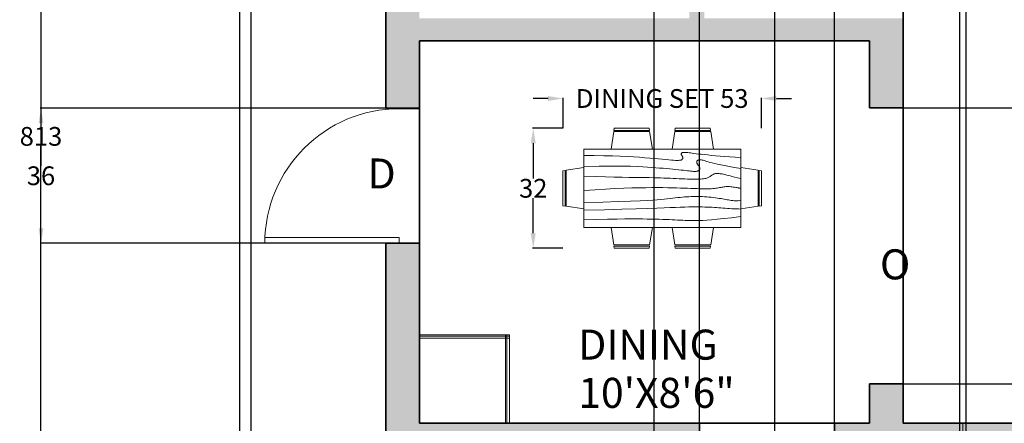
# Model space of a CAD drawing. Units: inches. Extents: x 460 to 1030, y -658 to 271.
# Tile 3 of 10: x 465 to 728, y -282 to -174. Entities that reach past the tile are written whole.
import ezdxf

# ---------------------------------------------------------------- set-up
doc = ezdxf.new("R2010")
doc.units = ezdxf.units.IN
doc.header["$MEASUREMENT"] = 0
for name, color, linetype, lineweight in [('A-ANNO-DIMS', 2, 'Continuous', 18), ('A-ANNO-TEXT', 7, 'Continuous', 18), ('A-AREA-IDEN', 7, 'Continuous', 25), ('A-DOOR', 3, 'Continuous', 20), ('A-FLOR-CASE', 9, 'Continuous', 18), ('A-FURN', 8, 'Continuous', 18), ('A-GLAZ', 4, 'Continuous', 20), ('A-GLAZ-PATT', 4, 'Continuous', 13), ('A-WALL', 7, 'Continuous', 35), ('A-WALL-PATT', 5, 'Continuous', 13), ('C-PROP', 7, 'Continuous', 25)]:
    doc.layers.add(name, color=color, linetype=linetype, lineweight=lineweight)
doc.styles.get("Standard").update_dxf_attribs({"font": 'arial.ttf'})
doc.dimstyles.get("Standard").update_dxf_attribs({"dimtxt": 5, "dimasz": 4, "dimexe": 0.18, "dimexo": 0.0625, "dimgap": 0.09, "dimtad": 0, "dimtih": 1, "dimtoh": 1, "dimdec": 1, "dimzin": 0, "dimdsep": 46, "dimlunit": 4, "dimtxsty": 'Standard', "dimcen": 0.09, "dimadec": 0, "dimazin": 0, "dimtfac": 1, "dimtdec": 1, "dimtofl": 0, "dimtmove": 0, "dimatfit": 3, "dimfxl": 1, "dimtolj": 1, "dimtzin": 0, "dimarcsym": 0})

# ---------------------------------------------------------------- blocks, each defined once
blk = doc.blocks.new('*U2')
for p, q in [((0, 0), (0, -6)), ((40, 0), (40, -6))]:
    blk.add_line(p, q)
blk.add_lwpolyline([(0, 0), (0, 40), (1.75, 40), (1.75, 0)], close=True)
blk.add_arc((0, 0), 40, 0, 90)
blk = doc.blocks.new('Dining Set - 36 x 72 in.')
for p, q in [((-22, 27.5), (-22.1562, 26.50042)), ((-22, 27.5), (-6, 27.5)), ((-5.8437, 26.49966), (-6, 27.5)), ((6, 27.5), (5.8438, 26.50042)), ((6, 27.5), (22, 27.5)), ((22.1563, 26.49966), (22, 27.5)), ((-22.2343, 26.00059), (-23.4847, 17.99762)), ((-22.2304, 26), (-5.7608, 26)), ((-5.8416, 26.5), (-22.1534, 26.5)), ((-4.5152, 17.99762), (-5.7655, 25.99926)), ((5.7657, 26.00059), (4.5153, 17.99762)), ((5.7696, 26), (22.2392, 26)), ((22.1584, 26.5), (5.8466, 26.5)), ((23.4848, 17.99762), (22.2345, 25.99926)), ((36, 18), (-36, 18)), ((-36, 18), (-36, -18)), ((36, -18), (36, 18)), ((-44.0006, 8.23428), (-35.9976, 9.48474)), ((44.0006, 8.23428), (35.9976, 9.48474)), ((-45.5, 8), (-44.5004, 8.15617)), ((-45.5, 8), (-45.5, -8)), ((-44.5, -8.15843), (-44.5, 8.15338)), ((-44, 8.23041), (-44, -8.23915)), ((44, 8.23041), (44, -8.23915)), ((44.5, -8.15843), (44.5, 8.15338)), ((45.5, 8), (44.5005, 8.15617)), ((45.5, 8), (45.5, -8)), ((-44.4997, -8.15631), (-45.5, -8)), ((-35.9976, -9.48476), (-43.9993, -8.2345)), ((35.9976, -9.48476), (43.9993, -8.2345)), ((44.4997, -8.15631), (45.5, -8)), ((-36, -18), (36, -18)), ((-22.2343, -26.0006), (-23.4847, -17.99762)), ((-4.5152, -17.99762), (-5.7655, -25.99928)), ((5.7657, -26.0006), (4.5153, -17.99762)), ((23.4848, -17.99762), (22.2345, -25.99928)), ((-22.2304, -26), (-5.7608, -26)), ((-22, -27.5), (-22.1562, -26.50044)), ((-5.8416, -26.5), (-22.1534, -26.5)), ((-5.8437, -26.49967), (-6, -27.5)), ((5.7696, -26), (22.2392, -26)), ((6, -27.5), (5.8438, -26.50044)), ((22.1584, -26.5), (5.8466, -26.5)), ((22.1563, -26.49967), (22, -27.5)), ((-22, -27.5), (-6, -27.5)), ((6, -27.5), (22, -27.5))]:
    blk.add_line(p, q)
for points in [[(-36, 15), (-31.1772, 14.97754), (-26.8079, 14.91406), (-22.8538, 14.81543), (-19.276, 14.6875), (-16.0362, 14.53613), (-13.0957, 14.36718), (-10.4159, 14.18652), (-7.9583, 14), (-5.6904, 13.81315), (-3.6035, 13.63021), (-1.6954, 13.45508), (0.0365, 13.29166), (1.5945, 13.14388), (2.9811, 13.01562), (4.1988, 12.9108), (5.25, 12.83333), (6.1393, 12.78613), (6.8802, 12.76823), (7.4883, 12.77767), (7.9792, 12.8125), (8.3685, 12.87077), (8.6719, 12.95052), (8.9049, 13.0498), (9.0833, 13.16666), (9.2205, 13.29899), (9.3216, 13.44401), (9.3895, 13.59879), (9.4271, 13.76041), (9.4373, 13.92594), (9.4232, 14.09245), (9.3875, 14.257), (9.3333, 14.41666), (9.2638, 14.56917), (9.1836, 14.71484), (9.0975, 14.85465), (9.0104, 14.98958), (8.9272, 15.1206), (8.8529, 15.2487), (8.7922, 15.37483), (8.75, 15.5), (8.7305, 15.62467), (8.7344, 15.74739), (8.7617, 15.86621), (8.8125, 15.97916), (8.8867, 16.08431), (8.9844, 16.17968), (9.1055, 16.26334), (9.25, 16.33333), (9.4189, 16.38802), (9.6172, 16.42708), (9.8506, 16.45052), (10.125, 16.45833), (10.4463, 16.45052), (10.8203, 16.42708), (11.2529, 16.38802), (11.75, 16.33333), (12.3184, 16.26318), (12.9694, 16.17838), (13.7151, 16.07991), (14.5677, 15.96875), (15.5395, 15.84586), (16.6426, 15.71224), (17.8893, 15.56884), (19.2917, 15.41666), (20.859, 15.25667), (22.5879, 15.08984), (24.4721, 14.91715), (26.5052, 14.73958), (28.6809, 14.5581), (30.9929, 14.3737), (33.4347, 14.18733), (36, 14)], [(-36, 10), (-28.9766, 10.14274), (-23.1725, 10.20442), (-18.4241, 10.19775), (-14.5677, 10.13541), (-11.4399, 10.03011), (-8.877, 9.89453), (-6.7154, 9.74137), (-4.7917, 9.58333), (-2.9698, 9.43082), (-1.2246, 9.28515), (0.4415, 9.14534), (2.026, 9.01041), (3.5266, 8.87939), (4.9408, 8.7513), (6.266, 8.62516), (7.5, 8.5), (8.6411, 8.37549), (9.6914, 8.2539), (10.6538, 8.13818), (11.5312, 8.03125), (12.3267, 7.93603), (13.043, 7.85547), (13.6831, 7.79248), (14.25, 7.75), (14.7471, 7.7303), (15.1797, 7.73307), (15.5537, 7.75732), (15.875, 7.80208), (16.1494, 7.86637), (16.3828, 7.94922), (16.5811, 8.04964), (16.75, 8.16666), (16.8944, 8.29915), (17.0143, 8.44531), (17.1089, 8.60319), (17.1771, 8.77083), (17.218, 8.94629), (17.2305, 9.1276), (17.2137, 9.31282), (17.1667, 9.5), (17.0895, 9.6875), (16.987, 9.875), (16.8649, 10.0625), (16.7292, 10.25), (16.5856, 10.4375), (16.4401, 10.625), (16.2985, 10.8125), (16.1667, 11), (16.05, 11.18733), (15.9518, 11.3737), (15.8752, 11.5581), (15.8229, 11.73958), (15.798, 11.91715), (15.8034, 12.08984), (15.842, 12.25667), (15.9167, 12.41666), (16.0295, 12.56836), (16.1784, 12.70833), (16.3605, 12.83268), (16.5729, 12.9375), (16.8127, 13.01888), (17.0768, 13.07291), (17.3625, 13.0957), (17.6667, 13.08333), (17.9894, 13.03312), (18.3418, 12.94726), (18.7382, 12.82918), (19.1927, 12.68229), (19.7195, 12.51001), (20.3327, 12.31575), (21.0465, 12.10294), (21.875, 11.875), (22.8357, 11.63354), (23.959, 11.37304), (25.2786, 11.08618), (26.8282, 10.76562), (28.6414, 10.40405), (30.752, 9.99414), (33.1936, 9.52856), (36, 9)], [(-36, 5.5), (-30.7157, 5.3348), (-26.069, 5.20963), (-21.9946, 5.11767), (-18.4271, 5.05208), (-15.3009, 5.00602), (-12.5508, 4.97265), (-10.1112, 4.94515), (-7.9167, 4.91666), (-5.909, 4.88167), (-4.0586, 4.83984), (-2.3429, 4.79215), (-0.7396, 4.73958), (0.7739, 4.6831), (2.22, 4.6237), (3.6213, 4.56233), (5, 4.5), (6.373, 4.43782), (7.7344, 4.3776), (9.0723, 4.32129), (10.375, 4.27083), (11.6309, 4.22819), (12.8281, 4.19531), (13.9551, 4.17415), (15, 4.16666), (15.954, 4.17448), (16.819, 4.19791), (17.6001, 4.23698), (18.3021, 4.29166), (18.9299, 4.36198), (19.4883, 4.44791), (19.9823, 4.54948), (20.4167, 4.66666), (20.7969, 4.79899), (21.1302, 4.94401), (21.4245, 5.09879), (21.6875, 5.26041), (21.9271, 5.42594), (22.1511, 5.59245), (22.3672, 5.757), (22.5834, 5.91666), (22.8065, 6.06868), (23.0404, 6.21093), (23.2879, 6.34147), (23.5521, 6.45833), (23.8358, 6.55957), (24.142, 6.64323), (24.4735, 6.70735), (24.8334, 6.75), (25.2235, 6.76969), (25.642, 6.76692), (26.0858, 6.74267), (26.5521, 6.69791), (27.0379, 6.63362), (27.5404, 6.55078), (28.0565, 6.45036), (28.5834, 6.33333), (29.1242, 6.19987), (29.7071, 6.04687), (30.3661, 5.87044), (31.1354, 5.66666), (32.0493, 5.43164), (33.142, 5.16146), (34.4475, 4.85221), (36, 4.5)], [(-36, -1), (-30.7915, -0.6591), (-26.0195, -0.38216), (-21.6519, -0.16284), (-17.6563, 0.00521), (-14.0005, 0.12833), (-10.6523, 0.21289), (-7.5796, 0.26522), (-4.75, 0.29166), (-2.134, 0.29793), (0.2878, 0.28711), (2.5317, 0.26163), (4.6146, 0.22396), (6.5529, 0.17651), (8.3633, 0.12174), (10.0623, 0.06209), (11.6667, 0), (13.1899, -0.06201), (14.6341, -0.1211), (15.9982, -0.17432), (17.2813, -0.21875), (18.4823, -0.25147), (19.6003, -0.26953), (20.6343, -0.27002), (21.5834, -0.25), (22.4481, -0.20768), (23.2357, -0.14584), (23.9549, -0.06836), (24.6146, 0.02083), (25.2235, 0.11784), (25.7904, 0.21875), (26.3241, 0.31966), (26.8334, 0.41666), (27.3265, 0.50618), (27.8099, 0.58593), (28.2894, 0.65397), (28.7709, 0.70833), (29.2601, 0.74707), (29.763, 0.76823), (30.2855, 0.76985), (30.8334, 0.75), (31.4088, 0.70784), (31.9994, 0.64713), (32.589, 0.57275), (33.1615, 0.48958), (33.7008, 0.4025), (34.1908, 0.3164), (34.6153, 0.23616), (34.9584, 0.16666), (35.2099, 0.11165), (35.3848, 0.07031), (35.504, 0.04069), (35.5886, 0.02083), (35.6594, 0.00879), (35.7377, 0.0026), (35.8442, 0.00032), (36, 0)], [(-36, -6.5), (-27.1843, -6.31267), (-20.084, -6.1263), (-14.469, -5.9419), (-10.1094, -5.76042), (-6.7752, -5.58285), (-4.2363, -5.41016), (-2.2629, -5.24333), (-0.625, -5.08334), (0.8708, -4.93099), (2.2715, -4.78646), (3.5872, -4.64974), (4.8281, -4.52084), (6.0046, -4.39974), (7.127, -4.28646), (8.2053, -4.18099), (9.25, -4.08334), (10.2705, -3.99382), (11.2734, -3.91407), (12.2647, -3.84603), (13.25, -3.79167), (14.2354, -3.75293), (15.2266, -3.73177), (16.2295, -3.73015), (17.25, -3.75), (18.2912, -3.79248), (19.3451, -3.85547), (20.4009, -3.93604), (21.4479, -4.03125), (22.4754, -4.13819), (23.4727, -4.25391), (24.4289, -4.37549), (25.3334, -4.5), (26.1785, -4.62492), (26.9694, -4.74935), (27.7145, -4.87281), (28.4219, -4.99479), (29.1, -5.11483), (29.7572, -5.23242), (30.4016, -5.34709), (31.0417, -5.45834), (31.6837, -5.56437), (32.3262, -5.65821), (32.9658, -5.73153), (33.599, -5.77604), (34.2224, -5.78345), (34.8327, -5.74545), (35.4264, -5.65373), (36, -5.5)], [(-36, -10), (-26.4022, -9.81299), (-18.4675, -9.62891), (-11.9839, -9.45069), (-6.7396, -9.28125), (-2.5226, -9.12354), (0.8789, -8.98047), (3.6769, -8.85498), (6.0833, -8.75), (8.2767, -8.66765), (10.3021, -8.60677), (12.1712, -8.56543), (13.8958, -8.54167), (15.4876, -8.53353), (16.9583, -8.53907), (18.3197, -8.55632), (19.5834, -8.58334), (20.7616, -8.61841), (21.8685, -8.66081), (22.9188, -8.71004), (23.9271, -8.76563), (24.9081, -8.82707), (25.8763, -8.89388), (26.8465, -8.96558), (27.8334, -9.04167), (28.8474, -9.12118), (29.8828, -9.20117), (30.93, -9.27824), (31.9792, -9.34896), (33.0205, -9.40991), (34.0443, -9.45768), (35.0407, -9.48885), (36, -9.5)], [(-36, -14.5), (-30.0881, -14.33513), (-25.0332, -14.21224), (-20.7312, -14.12647), (-17.0781, -14.07292), (-13.97, -14.04671), (-11.3027, -14.04297), (-8.9724, -14.05681), (-6.875, -14.08334), (-4.9224, -14.11833), (-3.0905, -14.16016), (-1.3709, -14.20785), (0.2448, -14.26042), (1.7647, -14.3169), (3.1973, -14.3763), (4.5507, -14.43767), (5.8333, -14.5), (7.0554, -14.5621), (8.235, -14.62175), (9.3922, -14.67652), (10.5469, -14.72396), (11.7192, -14.76164), (12.929, -14.78711), (14.1965, -14.79794), (15.5417, -14.79167), (16.9933, -14.76424), (18.6152, -14.70508), (20.4804, -14.60197), (22.6615, -14.44271), (25.2312, -14.21509), (28.2624, -13.9069), (31.8277, -13.50594), (36, -13)]]:
    blk.add_lwpolyline(points)
blk = doc.blocks.new('*D35')
at = {"layer": 'A-ANNO-DIMS', "color": 0, "lineweight": -2, "transparency": 16777216}
for p, q in [((606.08, -195.13), (602.08, -195.13)), ((610.08, -203.01), (610.08, -194.95)), ((663, -203.01), (663, -194.95)), ((667, -195.13), (671, -195.13))]:
    blk.add_line(p, q, dxfattribs=at)
at = {"layer": 'A-ANNO-DIMS', "color": 0, "transparency": 16777216}
for points in [[(606.08, -194.47), (606.08, -195.8), (610.08, -195.13)], [(667, -194.47), (667, -195.8), (663, -195.13)]]:
    blk.add_solid(points, dxfattribs=at)
at = {"layer": 'Defpoints', "color": 0, "transparency": 16777216}
for p in [(663, -195.13), (610.08, -203.07), (663, -203.07)]:
    blk.add_point(p, dxfattribs=at)
at = {"layer": 'A-ANNO-DIMS', "color": 0, "transparency": 16777216, "insert": (636.54, -195.13), "char_height": 5, "attachment_point": 5}
blk.add_mtext('\\A1;DINING SET 53', dxfattribs=at)
blk = doc.blocks.new('*D36')
at = {"layer": 'A-ANNO-DIMS', "color": 0, "lineweight": -2, "transparency": 16777216}
for p, q in [((610.02, -203.07), (601.96, -203.07)), ((602.14, -207.07), (602.14, -216.42)), ((602.14, -231.06), (602.14, -221.71)), ((610.02, -235.06), (601.96, -235.06))]:
    blk.add_line(p, q, dxfattribs=at)
at = {"layer": 'A-ANNO-DIMS', "color": 0, "transparency": 16777216}
for points in [[(601.47, -207.07), (602.81, -207.07), (602.14, -203.07)], [(601.47, -231.06), (602.81, -231.06), (602.14, -235.06)]]:
    blk.add_solid(points, dxfattribs=at)
at = {"layer": 'Defpoints', "color": 0, "transparency": 16777216}
for p in [(602.14, -203.07), (610.08, -203.07), (610.08, -235.06)]:
    blk.add_point(p, dxfattribs=at)
at = {"layer": 'A-ANNO-DIMS', "color": 0, "transparency": 16777216, "insert": (602.14, -219.07), "char_height": 5, "attachment_point": 5}
blk.add_mtext('\\A1;32', dxfattribs=at)
blk = doc.blocks.new('*D40')
at = {"layer": 'A-ANNO-DIMS', "color": 0, "lineweight": -2, "transparency": 16777216}
for p, q in [((523.73, 201.27), (470.68, 201.27)), ((470.86, 197.27), (470.86, -202.58)), ((470.86, -607.73), (470.86, -207.87)), ((523.73, -611.73), (470.68, -611.73))]:
    blk.add_line(p, q, dxfattribs=at)
at = {"layer": 'A-ANNO-DIMS', "color": 0, "transparency": 16777216}
for points in [[(470.19, 197.27), (471.52, 197.27), (470.86, 201.27)], [(470.19, -607.73), (471.52, -607.73), (470.86, -611.73)]]:
    blk.add_solid(points, dxfattribs=at)
at = {"layer": 'Defpoints', "color": 0, "transparency": 16777216}
for p in [(470.86, 201.27), (523.8, 201.27), (523.8, -611.73)]:
    blk.add_point(p, dxfattribs=at)
at = {"layer": 'A-ANNO-DIMS', "color": 0, "transparency": 16777216, "insert": (470.86, -205.23), "char_height": 5, "attachment_point": 5}
blk.add_mtext('\\A1;813', dxfattribs=at)
blk = doc.blocks.new('*D57')
at = {"layer": 'A-ANNO-DIMS', "color": 0, "lineweight": -2, "transparency": 16777216}
for p, q in [((717.53, -38.79), (717.53, -654.61)), ((741.59, -38.79), (741.59, -654.61)), ((713.53, -654.43), (709.53, -654.43)), ((745.59, -654.43), (749.59, -654.43))]:
    blk.add_line(p, q, dxfattribs=at)
at = {"layer": 'A-ANNO-DIMS', "color": 0, "transparency": 16777216}
for points in [[(713.53, -653.77), (713.53, -655.1), (717.53, -654.43)], [(745.59, -653.77), (745.59, -655.1), (741.59, -654.43)]]:
    blk.add_solid(points, dxfattribs=at)
at = {"layer": 'Defpoints', "color": 0, "transparency": 16777216}
for p in [(717.53, -38.73), (741.59, -38.73), (741.59, -654.43)]:
    blk.add_point(p, dxfattribs=at)
at = {"layer": 'A-ANNO-DIMS', "color": 0, "transparency": 16777216, "insert": (729.56, -654.43), "char_height": 5, "attachment_point": 5}
blk.add_mtext('\\A1;24.065', dxfattribs=at)
blk = doc.blocks.new('*D61')
at = {"layer": 'A-ANNO-DIMS', "color": 0, "lineweight": -2, "transparency": 16777216}
for p, q in [((646.47, -287.66), (646.47, 267.89)), ((682.47, -287.66), (682.47, 267.89)), ((650.47, 267.71), (660.81, 267.71)), ((678.47, 267.71), (668.14, 267.71))]:
    blk.add_line(p, q, dxfattribs=at)
at = {"layer": 'A-ANNO-DIMS', "color": 0, "transparency": 16777216}
for points in [[(650.47, 268.38), (650.47, 267.04), (646.47, 267.71)], [(678.47, 268.38), (678.47, 267.04), (682.47, 267.71)]]:
    blk.add_solid(points, dxfattribs=at)
at = {"layer": 'Defpoints', "color": 0, "transparency": 16777216}
for p in [(682.47, 267.71), (646.47, -287.73), (682.47, -287.73)]:
    blk.add_point(p, dxfattribs=at)
at = {"layer": 'A-ANNO-DIMS', "color": 0, "transparency": 16777216, "insert": (664.47, 267.71), "char_height": 5, "attachment_point": 5}
blk.add_mtext('\\A1;36', dxfattribs=at)
blk = doc.blocks.new('*D62')
at = {"layer": 'A-ANNO-DIMS', "color": 0, "lineweight": -2, "transparency": 16777216}
for p, q in [((700.86, -197.58), (1022.03, -197.58)), ((1021.85, -201.58), (1021.85, -231.74)), ((1021.85, -267.2), (1021.85, -237.03)), ((700.86, -271.2), (1022.03, -271.2))]:
    blk.add_line(p, q, dxfattribs=at)
at = {"layer": 'A-ANNO-DIMS', "color": 0, "transparency": 16777216}
for points in [[(1021.18, -201.58), (1022.51, -201.58), (1021.85, -197.58)], [(1021.18, -267.2), (1022.51, -267.2), (1021.85, -271.2)]]:
    blk.add_solid(points, dxfattribs=at)
at = {"layer": 'Defpoints', "color": 0, "transparency": 16777216}
for p in [(700.8, -197.58), (700.8, -271.2), (1021.85, -271.2)]:
    blk.add_point(p, dxfattribs=at)
at = {"layer": 'A-ANNO-DIMS', "color": 0, "transparency": 16777216, "insert": (1021.85, -234.39), "char_height": 5, "attachment_point": 5}
blk.add_mtext('\\A1;73.62', dxfattribs=at)
blk = doc.blocks.new('*D64')
at = {"layer": 'A-ANNO-DIMS', "color": 0, "lineweight": -2, "transparency": 16777216}
for p, q in [((562.73, -197.73), (470.68, -197.73)), ((470.86, -201.73), (470.86, -213.08)), ((470.86, -229.73), (470.86, -218.37)), ((562.73, -233.73), (470.68, -233.73))]:
    blk.add_line(p, q, dxfattribs=at)
at = {"layer": 'A-ANNO-DIMS', "color": 0, "transparency": 16777216}
for points in [[(470.19, -201.73), (471.52, -201.73), (470.86, -197.73)], [(470.19, -229.73), (471.52, -229.73), (470.86, -233.73)]]:
    blk.add_solid(points, dxfattribs=at)
at = {"layer": 'Defpoints', "color": 0, "transparency": 16777216}
for p in [(562.8, -197.73), (470.86, -233.73), (562.8, -233.73)]:
    blk.add_point(p, dxfattribs=at)
at = {"layer": 'A-ANNO-DIMS', "color": 0, "transparency": 16777216, "insert": (470.86, -215.73), "char_height": 5, "attachment_point": 5}
blk.add_mtext('\\A1;36', dxfattribs=at)
blk = doc.blocks.new('*D68')
at = {"layer": 'A-ANNO-DIMS', "color": 0, "lineweight": -2, "transparency": 16777216}
for p, q in [((634.27, 90.21), (634.27, -654.61)), ((666.46, 90.21), (666.46, -654.61)), ((638.27, -654.43), (639.91, -654.43)), ((662.46, -654.43), (660.82, -654.43))]:
    blk.add_line(p, q, dxfattribs=at)
at = {"layer": 'A-ANNO-DIMS', "color": 0, "transparency": 16777216}
for points in [[(638.27, -653.77), (638.27, -655.1), (634.27, -654.43)], [(662.46, -653.77), (662.46, -655.1), (666.46, -654.43)]]:
    blk.add_solid(points, dxfattribs=at)
at = {"layer": 'Defpoints', "color": 0, "transparency": 16777216}
for p in [(634.27, 90.27), (666.46, 90.27), (666.46, -654.43)]:
    blk.add_point(p, dxfattribs=at)
at = {"layer": 'A-ANNO-DIMS', "color": 0, "transparency": 16777216, "insert": (650.37, -654.43), "char_height": 5, "attachment_point": 5}
blk.add_mtext('\\A1;32.184', dxfattribs=at)
blk = doc.blocks.new('*D72')
at = {"layer": 'A-ANNO-DIMS', "color": 0, "lineweight": -2, "transparency": 16777216}
for p, q in [((715.8, 68.25), (715.8, -654.61)), ((748.8, 57.75), (748.8, -654.61)), ((719.8, -654.43), (728.63, -654.43)), ((744.8, -654.43), (735.97, -654.43))]:
    blk.add_line(p, q, dxfattribs=at)
at = {"layer": 'A-ANNO-DIMS', "color": 0, "transparency": 16777216}
for points in [[(719.8, -653.77), (719.8, -655.1), (715.8, -654.43)], [(744.8, -653.77), (744.8, -655.1), (748.8, -654.43)]]:
    blk.add_solid(points, dxfattribs=at)
at = {"layer": 'Defpoints', "color": 0, "transparency": 16777216}
for p in [(715.8, 68.31), (748.8, 57.81), (748.8, -654.43)]:
    blk.add_point(p, dxfattribs=at)
at = {"layer": 'A-ANNO-DIMS', "color": 0, "transparency": 16777216, "insert": (732.3, -654.43), "char_height": 5, "attachment_point": 5}
blk.add_mtext('\\A1;33', dxfattribs=at)

msp = doc.modelspace()

# ---------------------------------------------------------------- hatches: boundary and pattern name
at = {"layer": 'A-GLAZ-PATT'}
h = msp.add_hatch(color=256, dxfattribs=at)
h.dxf.hatch_style = 1
h.paths.add_polyline_path([(571.7961, -343.9041), (562.7961, -343.9041), (562.7961, -384.3969), (571.7961, -384.3969)])
h.paths.add_polyline_path([(571.7961, -143.2895), (562.7961, -143.2895), (562.7961, -168.3798), (571.7961, -168.3798)])
h.paths.add_polyline_path([(571.7961, -49.2966), (562.7961, -49.2966), (562.7961, -90.3192), (571.7961, -90.3192)])
h.paths.add_polyline_path([(666.4584, 90.2738), (634.2742, 90.2738), (634.2742, 81.2738), (666.4584, 81.2738)])
h.paths.add_polyline_path([(742.1779, 90.2738), (713.201, 90.2738), (713.201, 81.2738), (742.1779, 81.2738)])
h.paths.add_polyline_path([(797.2395, 90.2738), (768.2626, 90.2738), (768.2626, 81.2738), (797.2395, 81.2738)])
h.paths.add_polyline_path([(918.7723, 90.2738), (881.2728, 90.2738), (881.2728, 81.2738), (918.7723, 81.2738)])
h.paths.add_polyline_path([(940.7961, -60.0042), (931.7961, -60.0042), (931.7961, -95.7262), (940.7961, -95.7262)])
h.paths.add_polyline_path([(940.7961, -163.6558), (931.7961, -163.6558), (931.7961, -230.2946), (940.7961, -230.2946)])
h.paths.add_polyline_path([(913.7961, -331.7262), (835.7961, -331.7262), (835.7961, -332.7262), (913.7961, -332.7262)])
h.paths.add_polyline_path([(871.4559, -281.7262), (831.4302, -281.7262), (831.4302, -287.7262), (871.4559, -287.7262)])
h.paths.add_polyline_path([(774.8576, -281.7262), (716.7073, -281.7262), (716.7073, -287.7262), (774.8576, -287.7262)])
at = {"layer": 'A-WALL-PATT'}
h = msp.add_hatch(color=256, dxfattribs=at)
h.dxf.hatch_style = 1
h.paths.add_polyline_path([(634.2742, 90.2738), (571.7961, 90.2738), (571.7961, 81.2738), (634.2742, 81.2738)])
h.paths.add_polyline_path([(691.7961, 90.2738), (666.4584, 90.2738), (666.4584, 81.2738), (691.7961, 81.2738)])
h.paths.add_polyline_path([(713.201, 90.2738), (700.7961, 90.2738), (700.7961, 81.2738), (713.201, 81.2738)])
h.paths.add_polyline_path([(748.7961, 90.2738), (742.1779, 90.2738), (742.1779, 81.2738), (748.7961, 81.2738)])
h.paths.add_polyline_path([(768.2626, 90.2738), (754.7961, 90.2738), (754.7961, 81.2738), (768.2626, 81.2738)])
h.paths.add_polyline_path([(802.7961, 90.2738), (797.2395, 90.2738), (797.2395, 81.2738), (802.7961, 81.2738)])
h.paths.add_polyline_path([(881.2728, 90.2738), (811.7961, 90.2738), (811.7961, 81.2738), (881.2728, 81.2738)])
h.paths.add_polyline_path([(931.7961, 90.2738), (918.7723, 90.2738), (918.7723, 81.2738), (931.7961, 81.2738)])
h.paths.add_polyline_path([(940.7961, 71.6966), (931.7961, 71.6966), (931.7961, -60.0042), (940.7961, -60.0042)])
h.paths.add_polyline_path([(940.7961, -95.7262), (931.7961, -95.7262), (931.7961, -101.149), (940.7961, -101.149)])
h.paths.add_polyline_path([(931.7961, -110.7262), (894.6225, -110.7262), (894.6225, -119.7262), (931.7961, -119.7262)])
h.paths.add_polyline_path([(858.6225, -110.7262), (811.7961, -110.7262), (811.7961, -119.7262), (858.6225, -119.7262)])
h.paths.add_polyline_path([(940.7961, -119.7262), (931.7961, -119.7262), (931.7961, -141.7212), (931.7961, -163.6558), (940.7961, -163.6558)])
h.paths.add_polyline_path([(940.7961, -230.2946), (931.7961, -230.2946), (931.7961, -268.3723), (940.7961, -268.3723)])
h.paths.add_polyline_path([(931.7961, -281.7262), (908.3452, -281.7262), (908.3452, -285.0181), (908.3452, -287.7262), (931.7961, -287.7262)])
h.paths.add_polyline_path([(831.4302, -281.7262), (803.0275, -281.7262), (803.0275, -287.7262), (808.7961, -287.7262), (808.7961, -339.7262), (811.7961, -339.7262), (811.7961, -287.7262), (831.4302, -287.7262)])
h.paths.add_polyline_path([(789.8237, -281.7262), (774.8576, -281.7262), (774.8576, -287.7262), (789.8237, -287.7262)])
h.paths.add_polyline_path([(716.7073, -281.7262), (700.7961, -281.7262), (700.7961, -271.1977), (691.7961, -271.1977), (691.7961, -281.7262), (682.4735, -281.7262), (682.4735, -287.7262), (691.7961, -287.7262), (691.7961, -303.809), (700.7961, -303.809), (700.7961, -287.7262), (716.7073, -287.7262)])
h.paths.add_polyline_path([(700.7961, -323.8443), (691.7961, -323.8443), (691.7961, -413.1453), (700.7961, -413.1453)])
h.paths.add_polyline_path([(940.7961, -287.7262), (937.7961, -287.7262), (937.7961, -339.7262), (940.7961, -339.7262)])
h.paths.add_polyline_path([(937.7961, -336.7262), (811.7961, -336.7262), (811.7961, -339.7262), (937.7961, -339.7262)])
h.paths.add_polyline_path([(835.7961, -329.7262), (811.7961, -329.7262), (811.7961, -332.7262), (835.7961, -332.7262)])
h.paths.add_polyline_path([(937.7961, -329.7262), (913.7961, -329.7262), (913.7961, -332.7262), (937.7961, -332.7262)])
h.paths.add_polyline_path([(691.7961, -419.7262), (681.4044, -419.7262), (681.4044, -428.7262), (691.7961, -428.7262)])
h.paths.add_polyline_path([(691.7961, -476.7262), (571.7961, -476.7262), (571.7961, -485.7262), (691.7961, -485.7262)])
h.paths.add_polyline_path([(571.7961, -465.0348), (568.223, -465.0348), (562.7961, -465.0348), (562.7961, -476.7262), (571.7961, -476.7262)])
h.paths.add_polyline_path([(571.7961, -432.4659), (562.7961, -432.4659), (562.7961, -441.1912), (571.7961, -441.1912)])
h.paths.add_polyline_path([(571.7961, -384.3969), (562.7961, -384.3969), (562.7961, -413.1453), (571.7961, -413.1453)])
h.paths.add_polyline_path([(571.7961, -323.8443), (562.7961, -323.8443), (562.7961, -343.9041), (571.7961, -343.9041)])
h.paths.add_polyline_path([(571.7961, -287.7262), (646.4735, -287.7262), (646.4735, -281.7262), (571.7961, -281.7262), (571.7961, -258.1542), (571.7961, -233.7262), (566.4164, -233.7262), (562.7961, -233.7262), (562.7961, -303.809), (571.7961, -303.809)])
h.paths.add_polyline_path([(571.7961, -179.7262), (691.7961, -179.7262), (691.7961, -197.5753), (700.7961, -197.5753), (700.7961, -173.7262), (647.7961, -173.7262), (647.7961, -165.5723), (643.7961, -165.5723), (643.7961, -173.7262), (571.7961, -173.7262), (571.7961, -168.3798), (562.7961, -168.3798), (562.7961, -197.7262), (571.7961, -197.7262)])
h.paths.add_polyline_path([(647.7961, -110.7262), (571.7961, -110.7262), (571.7961, -119.7262), (643.7961, -119.7262), (643.7961, -141.5723), (647.7961, -141.5723)])
h.paths.add_polyline_path([(691.7961, -110.7262), (683.7961, -110.7262), (683.7961, -114.3453), (683.7961, -119.7262), (691.7961, -119.7262)])
h.paths.add_polyline_path([(571.7961, -119.7262), (562.7961, -119.7262), (562.7961, -143.2895), (571.7961, -143.2895)])
h.paths.add_polyline_path([(571.7961, -90.3192), (562.7961, -90.3192), (562.7961, -101.149), (571.7961, -101.149)])
h.paths.add_polyline_path([(571.7961, 71.6966), (562.7961, 71.6966), (562.7961, -49.2966), (571.7961, -49.2966)])
h.paths.add_polyline_path([(700.7961, 71.6966), (691.7961, 71.6966), (691.7961, -50.298), (700.7961, -50.298)])
h.paths.add_polyline_path([(754.7961, 81.2738), (748.7961, 81.2738), (748.7961, -38.7262), (741.5908, -38.7262), (741.5908, -39.109), (741.5908, -42.7262), (748.7961, -42.7262), (748.7961, -110.7262), (754.7961, -110.7262), (754.7961, -42.7262), (773.6274, -42.7262), (773.6274, -38.7262), (754.7961, -38.7262)])
h.paths.add_polyline_path([(717.4759, -38.7262), (700.7961, -38.7262), (700.7961, -42.7262), (717.4759, -42.7262)])
h.paths.add_polyline_path([(811.7961, 71.6966), (802.7961, 71.6966), (802.7961, -50.298), (811.7961, -50.298)])
h.paths.add_polyline_path([(811.7961, -86.298), (806.4164, -86.298), (802.7961, -86.298), (802.7961, -101.149), (811.7961, -101.149)])

# ---------------------------------------------------------------- linework, layer by layer
at = {"layer": 'A-FLOR-CASE'}
for p, q in [((571.7961, -258.4994), (595.7961, -258.4994)), ((571.7961, -258.9871), (595.7961, -258.9871)), ((594.7141, -258.1542), (594.7141, -281.7262)), ((595.084, -258.1542), (595.084, -281.7262))]:
    msp.add_line(p, q, dxfattribs=at)
msp.add_lwpolyline([(571.7961, -281.7262), (595.7961, -281.7262), (595.7961, -258.1542), (571.7961, -258.1542)], close=True, dxfattribs=at)
at = {"layer": 'A-GLAZ'}
msp.add_lwpolyline([(716.7073, -281.7262), (774.8576, -281.7262), (774.8576, -287.7262), (716.7073, -287.7262)], close=True, dxfattribs=at)
at = {"layer": 'A-WALL'}
for p, q in [((562.7961, 90.2738), (562.7961, -197.7262)), ((700.7961, -86.298), (700.7961, -281.7262)), ((691.7961, -179.7262), (571.7961, -179.7262)), ((571.7961, -179.7262), (571.7961, -197.7262)), ((691.7961, -179.7262), (691.7961, -197.5753)), ((562.7961, -197.7262), (571.7961, -197.7262)), ((571.7961, -197.7262), (571.7961, -281.7262)), ((691.7961, -197.5753), (700.7961, -197.5753)), ((571.7961, -233.7262), (562.7961, -233.7262)), ((562.7961, -233.7262), (562.7961, -441.1912)), ((700.7961, -271.1977), (691.7961, -271.1977)), ((691.7961, -271.1977), (691.7961, -281.7262)), ((691.7961, -271.1977), (691.7961, -281.7262)), ((691.7961, -281.7262), (571.7961, -281.7262)), ((646.4735, -287.7262), (646.4735, -281.7262)), ((682.4735, -281.7262), (682.4735, -287.7262)), ((872.2999, -281.7262), (700.7961, -281.7262))]:
    msp.add_line(p, q, dxfattribs=at)
at = {"layer": 'C-PROP'}
for p, q in [((523.7961, 129.2738), (523.7961, -524.7262)), ((526.7961, 126.2738), (526.7961, -608.7262))]:
    msp.add_line(p, q, dxfattribs=at)

# ---------------------------------------------------------------- block references
at = {"layer": 'A-DOOR', "xscale": 0.8966154602300187, "yscale": 0.8966154602300187, "zscale": 0.8966154602300187, "rotation": 90.00000000000003}
msp.add_blockref('*U2', (566.4164, -233.7262), dxfattribs=at)
at = {"layer": 'A-FURN', "xscale": 0.5816064749315994, "yscale": 0.5816064749315994, "zscale": 0.5816064749315994}
msp.add_blockref('Dining Set - 36 x 72 in.', (636.5409, -219.0672), dxfattribs=at)

# ---------------------------------------------------------------- texts
at = {"layer": 'A-ANNO-TEXT'}
for s, p in [('D', (557.9567, -219.1244)), ('O', (694.6119, -243.3472))]:
    msp.add_text(s, height=8, dxfattribs=at).set_placement(p)
at = {"layer": 'A-AREA-IDEN'}
for s, p in [('DINING', (614.1476, -264.757)), ('10\'X8\'6"', (614.1476, -277.6083))]:
    msp.add_text(s, height=8, dxfattribs=at).set_placement(p)

# ---------------------------------------------------------------- dimensions: what is measured, and where the dimension line sits
at = {"layer": 'A-ANNO-DIMS'}
for base, p1, p2, override, picture, middle in [((682.4735, 267.7108), (646.4735, -287.7262), (682.4735, -287.7262), {"dimdec": 0, "dimlfac": 1, "dimrnd": 0, "dimzin": 0, "dimdsep": 46, "dimlunit": 2}, '*D61', (664.4735, 267.7108)), ((666.4584, -654.4339), (634.2742, 90.2738), (666.4584, 90.2738), {"dimdec": 3, "dimlfac": 1, "dimrnd": 0, "dimzin": 0, "dimdsep": 46, "dimlunit": 2}, '*D68', (650.3663, -654.4339)), ((748.7961, -654.4339), (715.7961, 68.3148), (748.7961, 57.8148), {"dimdec": 0, "dimlfac": 1, "dimrnd": 0, "dimzin": 0, "dimdsep": 46, "dimlunit": 2}, '*D72', (732.2961, -654.4339)), ((741.5908, -654.4339), (717.5258, -38.7262), (741.5908, -38.7262), {"dimdec": 3, "dimlfac": 1, "dimrnd": 0, "dimzin": 0, "dimdsep": 46, "dimlunit": 2}, '*D57', (729.5583, -654.4339))]:
    dim = msp.add_linear_dim(base=base, p1=p1, p2=p2, dimstyle='Standard', override=override, dxfattribs=at)
    dim.commit()
    dim.dimension.update_dxf_attribs({"geometry": picture, "text_midpoint": middle})
for base, p1, p2, override, picture, middle in [((470.8563, 201.2738), (523.7961, -611.7262), (523.7961, 201.2738), {"dimdec": 0, "dimlfac": 1, "dimrnd": 0, "dimzin": 0, "dimdsep": 46, "dimlunit": 2}, '*D40', (470.8563, -205.2262)), ((470.8563, -233.7262), (562.7961, -197.7262), (562.7961, -233.7262), {"dimdec": 0, "dimlfac": 1, "dimrnd": 0, "dimzin": 0, "dimdsep": 46, "dimlunit": 2}, '*D64', (470.8563, -215.7262)), ((1021.8461, -271.1977), (700.7961, -197.5753), (700.7961, -271.1977), {"dimdec": 2, "dimlfac": 1, "dimrnd": 0, "dimzin": 0, "dimdsep": 46, "dimlunit": 2}, '*D62', (1021.8461, -234.3865)), ((602.1389, -203.073), (610.0778, -235.0614), (610.0778, -203.073), {"dimdec": 0, "dimlfac": 1, "dimrnd": 0, "dimzin": 0, "dimdsep": 46, "dimlunit": 2}, '*D36', (602.1389, -219.0672))]:
    dim = msp.add_linear_dim(base=base, p1=p1, p2=p2, angle=90, dimstyle='Standard', override=override, dxfattribs=at)
    dim.commit()
    dim.dimension.update_dxf_attribs({"geometry": picture, "text_midpoint": middle})
dim = msp.add_linear_dim(base=(663.004, -195.1341), p1=(610.0778, -203.073), p2=(663.004, -203.073), text='DINING SET <>', dimstyle='Standard', override={"dimdec": 0, "dimlfac": 1, "dimrnd": 0, "dimzin": 0, "dimdsep": 46, "dimlunit": 2}, dxfattribs=at)
dim.commit()
dim.dimension.update_dxf_attribs({"geometry": '*D35', "text_midpoint": (636.5409, -195.1341)})

doc.saveas('drawing.dxf')
